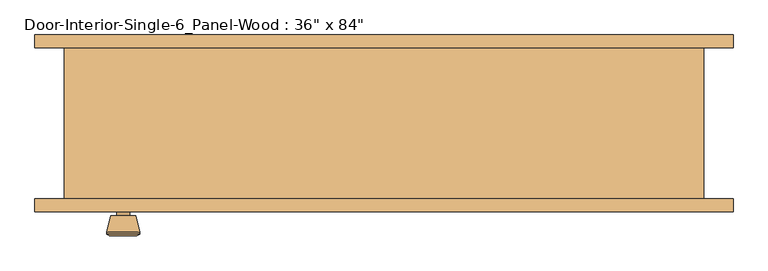
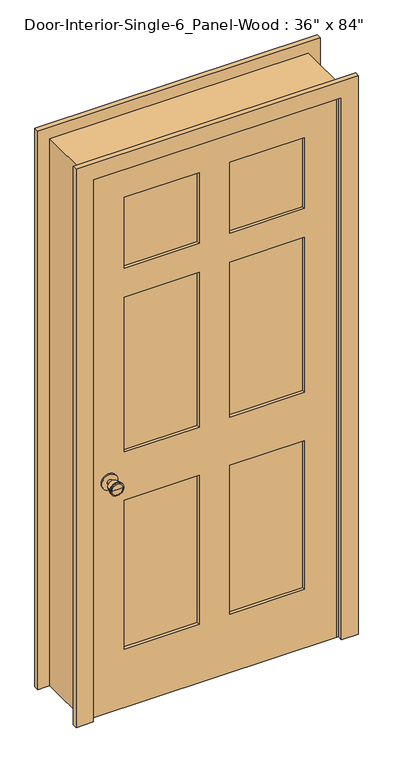
"""IFC4 building model written with IfcOpenShell, lengths in millimetres: door geometry."""

from ifc_helpers import new_model, si_unit, point, frame, frame_2d, origin, place, context, project, spatial, polyline, circle_curve, trimmed, segment, composite_curve, outline, extrude, faceted_brep, source, transform, mapped, element, save
from ifc_brep_helpers import plane_surface, cylinder_surface, revolved_surface, advanced_brep


def door_c5239341(model_context):
    return source(origin(), model_context, "Body", "SolidModel", [
        advanced_brep(
        [(-393.7, -70.2, 914.4), (-403.7, -70.2, 914.4), (-383.7, -70.2, 914.4), (-373.2241324, -21.2, 914.4), (-414.1758676, -21.2, 914.4), (-393.7, -21.2, 914.4), (-368.7, -23.0278681, 914.4), (-418.7, -23.0278681, 914.4), (-368.7, -26.4915463, 914.4), (-418.7, -26.4915463, 914.4), (-375.063764, -51.2, 914.4), (-412.336236, -51.2, 914.4), (-383.7, -51.2, 914.4), (-403.7, -51.2, 914.4)],
        [
            (0, 1),
            (1, 2, circle_curve(frame((-393.7, -70.2, 914.4), z_axis=(0.0, -1.0, 0.0), x_axis=(-1.0, 0.0, 0.0)), 10.0)),
            (2, 0),
            (2, 1, circle_curve(frame((-393.7, -70.2, 914.4), z_axis=(0.0, -1.0, 0.0), x_axis=(-1.0, 0.0, 0.0)), 10.0)),
            (3, 4, circle_curve(frame((-393.7, -21.2, 914.4), z_axis=(0.0, 1.0, 0.0), x_axis=(-1.0, 0.0, 0.0)), 20.4758676)),
            (4, 5),
            (5, 3),
            (4, 3, circle_curve(frame((-393.7, -21.2, 914.4), z_axis=(0.0, 1.0, 0.0), x_axis=(-1.0, 0.0, 0.0)), 20.4758676)),
            (6, 7, circle_curve(frame((-393.7, -23.0278681, 914.4), z_axis=(0.0, 1.0, 0.0), x_axis=(-1.0, 0.0, 0.0)), 25.0)),
            (7, 4),
            (3, 6),
            (7, 6, circle_curve(frame((-393.7, -23.0278681, 914.4), z_axis=(0.0, 1.0, 0.0), x_axis=(-1.0, 0.0, 0.0)), 25.0)),
            (8, 9, circle_curve(frame((-393.7, -26.4915463, 914.4), z_axis=(0.0, 1.0, 0.0), x_axis=(-1.0, 0.0, 0.0)), 25.0)),
            (9, 7),
            (6, 8),
            (9, 8, circle_curve(frame((-393.7, -26.4915463, 914.4), z_axis=(0.0, 1.0, 0.0), x_axis=(-1.0, 0.0, 0.0)), 25.0)),
            (10, 11, circle_curve(frame((-393.7, -51.2, 914.4), z_axis=(0.0, 1.0, 0.0), x_axis=(-1.0, 0.0, 0.0)), 18.636236)),
            (11, 9),
            (8, 10),
            (11, 10, circle_curve(frame((-393.7, -51.2, 914.4), z_axis=(0.0, 1.0, 0.0), x_axis=(-1.0, 0.0, 0.0)), 18.636236)),
            (12, 13, circle_curve(frame((-393.7, -51.2, 914.4), z_axis=(0.0, 1.0, 0.0), x_axis=(-1.0, 0.0, 0.0)), 10.0)),
            (13, 11),
            (10, 12),
            (13, 12, circle_curve(frame((-393.7, -51.2, 914.4), z_axis=(0.0, 1.0, 0.0), x_axis=(-1.0, 0.0, 0.0)), 10.0)),
            (1, 13),
            (12, 2),
        ],
        [
            plane_surface(frame((-393.7, -70.2, 914.4), z_axis=(0.0, -1.0, 0.0), x_axis=(-1.0, 0.0, 0.0))),
            plane_surface(frame((-393.7, -21.2, 914.4), z_axis=(0.0, 1.0, 0.0), x_axis=(-1.0, 0.0, 0.0))),
            revolved_surface(polyline([(-414.1758676, -21.2, 914.4), (-418.7, -23.0278681, 914.4)]), (-393.7, -70.2, 914.4), (0.0, -1.0, 0.0)),
            cylinder_surface(frame((-393.7, -70.2, 914.4), z_axis=(0.0, -1.0, 0.0), x_axis=(-1.0, 0.0, 0.0)), 25.0),
            revolved_surface(polyline([(-418.7, -26.4915463, 914.4), (-412.336236, -51.2, 914.4)]), (-393.7, -70.2, 914.4), (0.0, -1.0, 0.0)),
            plane_surface(frame((-393.7, -51.2, 914.4), z_axis=(0.0, -1.0, 0.0), x_axis=(-1.0, 0.0, 0.0))),
            cylinder_surface(frame((-393.7, -70.2, 914.4), z_axis=(0.0, -1.0, 0.0), x_axis=(-1.0, 0.0, 0.0)), 10.0),
        ],
        [
            (0, [[1, 2, 3]]),
            (0, [[-3, 4, -1]]),
            (1, [[5, 6, 7]]),
            (1, [[8, -7, -6]]),
            (2, [[9, 10, -5, 11]]),
            (2, [[12, -11, -8, -10]]),
            (3, [[13, 14, -9, 15]]),
            (3, [[16, -15, -12, -14]]),
            (4, [[17, 18, -13, 19]]),
            (4, [[20, -19, -16, -18]]),
            (5, [[21, 22, -17, 23]]),
            (5, [[24, -23, -20, -22]]),
            (6, [[-2, 25, -21, 26]]),
            (6, [[-4, -26, -24, -25]]),
        ],
    ),
        extrude(outline(composite_curve([segment(trimmed(circle_curve(frame_2d((914.4, -393.7)), 30.0), [point((914.4, -423.7))], [point((914.4, -363.7))], False, "CARTESIAN"), True, "CONTINUOUS"), segment(trimmed(circle_curve(frame_2d((914.4, -393.7)), 30.0), [point((914.4, -363.7))], [point((914.4, -423.7))], False, "CARTESIAN"), True, "CONTINUOUS")], self_intersect=False)), frame((0.0, -76.2, 0.0), z_axis=(0.0, 1.0, 0.0), x_axis=(0.0, 0.0, 1.0)), (0.0, 0.0, 1.0), 6.0),
        advanced_brep(
        [(-393.7, -117.125, 914.4), (-383.7, -117.125, 914.4), (-403.7, -117.125, 914.4), (-373.2241324, -166.125, 914.4), (-393.7, -166.125, 914.4), (-414.1758676, -166.125, 914.4), (-368.7, -164.2971319, 914.4), (-418.7, -164.2971319, 914.4), (-368.7, -160.8334537, 914.4), (-418.7, -160.8334537, 914.4), (-375.063764, -136.125, 914.4), (-412.336236, -136.125, 914.4), (-383.7, -136.125, 914.4), (-403.7, -136.125, 914.4)],
        [
            (0, 1),
            (1, 2, circle_curve(frame((-393.7, -117.125, 914.4), z_axis=(0.0, 1.0, 0.0), x_axis=(-1.0, 0.0, 0.0)), 10.0)),
            (2, 0),
            (2, 1, circle_curve(frame((-393.7, -117.125, 914.4), z_axis=(0.0, 1.0, 0.0), x_axis=(-1.0, 0.0, 0.0)), 10.0)),
            (3, 4),
            (4, 5),
            (5, 3, circle_curve(frame((-393.7, -166.125, 914.4), z_axis=(0.0, -1.0, 0.0), x_axis=(-1.0, 0.0, 0.0)), 20.4758676)),
            (3, 5, circle_curve(frame((-393.7, -166.125, 914.4), z_axis=(0.0, -1.0, 0.0), x_axis=(-1.0, 0.0, 0.0)), 20.4758676)),
            (6, 3),
            (5, 7),
            (7, 6, circle_curve(frame((-393.7, -164.2971319, 914.4), z_axis=(0.0, -1.0, 0.0), x_axis=(-1.0, 0.0, 0.0)), 25.0)),
            (6, 7, circle_curve(frame((-393.7, -164.2971319, 914.4), z_axis=(0.0, -1.0, 0.0), x_axis=(-1.0, 0.0, 0.0)), 25.0)),
            (8, 6),
            (7, 9),
            (9, 8, circle_curve(frame((-393.7, -160.8334537, 914.4), z_axis=(0.0, -1.0, 0.0), x_axis=(-1.0, 0.0, 0.0)), 25.0)),
            (8, 9, circle_curve(frame((-393.7, -160.8334537, 914.4), z_axis=(0.0, -1.0, 0.0), x_axis=(-1.0, 0.0, 0.0)), 25.0)),
            (10, 8),
            (9, 11),
            (11, 10, circle_curve(frame((-393.7, -136.125, 914.4), z_axis=(0.0, -1.0, 0.0), x_axis=(-1.0, 0.0, 0.0)), 18.636236)),
            (10, 11, circle_curve(frame((-393.7, -136.125, 914.4), z_axis=(0.0, -1.0, 0.0), x_axis=(-1.0, 0.0, 0.0)), 18.636236)),
            (12, 10),
            (11, 13),
            (13, 12, circle_curve(frame((-393.7, -136.125, 914.4), z_axis=(0.0, -1.0, 0.0), x_axis=(-1.0, 0.0, 0.0)), 10.0)),
            (12, 13, circle_curve(frame((-393.7, -136.125, 914.4), z_axis=(0.0, -1.0, 0.0), x_axis=(-1.0, 0.0, 0.0)), 10.0)),
            (1, 12),
            (13, 2),
        ],
        [
            plane_surface(frame((-393.7, -117.125, 914.4), z_axis=(0.0, 1.0, 0.0), x_axis=(-1.0, 0.0, 0.0))),
            plane_surface(frame((-393.7, -166.125, 914.4), z_axis=(0.0, -1.0, 0.0), x_axis=(-1.0, 0.0, 0.0))),
            revolved_surface(polyline([(-414.1758676, -166.125, 914.4), (-418.7, -164.2971319, 914.4)]), (-393.7, -117.125, 914.4), (0.0, 1.0, 0.0)),
            cylinder_surface(frame((-393.7, -117.125, 914.4), z_axis=(0.0, 1.0, 0.0), x_axis=(-1.0, 0.0, 0.0)), 25.0),
            revolved_surface(polyline([(-418.7, -160.8334537, 914.4), (-412.336236, -136.125, 914.4)]), (-393.7, -117.125, 914.4), (0.0, 1.0, 0.0)),
            plane_surface(frame((-393.7, -136.125, 914.4), z_axis=(0.0, 1.0, 0.0), x_axis=(-1.0, 0.0, 0.0))),
            cylinder_surface(frame((-393.7, -117.125, 914.4), z_axis=(0.0, 1.0, 0.0), x_axis=(-1.0, 0.0, 0.0)), 10.0),
        ],
        [
            (0, [[1, 2, 3]]),
            (0, [[-3, 4, -1]]),
            (1, [[5, 6, 7]]),
            (1, [[-6, -5, 8]]),
            (2, [[9, -7, 10, 11]]),
            (2, [[-10, -8, -9, 12]]),
            (3, [[13, -11, 14, 15]]),
            (3, [[-14, -12, -13, 16]]),
            (4, [[17, -15, 18, 19]]),
            (4, [[-18, -16, -17, 20]]),
            (5, [[21, -19, 22, 23]]),
            (5, [[-22, -20, -21, 24]]),
            (6, [[25, -23, 26, -2]]),
            (6, [[-26, -24, -25, -4]]),
        ],
    ),
        extrude(outline(composite_curve([segment(trimmed(circle_curve(frame_2d((914.4, -393.7)), 30.0), [point((914.4, -423.7))], [point((914.4, -363.7))], False, "CARTESIAN"), True, "CONTINUOUS"), segment(trimmed(circle_curve(frame_2d((914.4, -393.7)), 30.0), [point((914.4, -363.7))], [point((914.4, -423.7))], False, "CARTESIAN"), True, "CONTINUOUS")], self_intersect=False)), frame((0.0, -117.125, 0.0), z_axis=(0.0, 1.0, 0.0), x_axis=(0.0, 0.0, 1.0)), (0.0, 0.0, 1.0), 6.0),
        faceted_brep([(482.6, -111.125, 0.0), (457.2, -111.125, 0.0), (457.2, -76.2, 0.0), (444.5, -76.2, 0.0), (444.5, -41.275, 0.0), (457.2, -41.275, 0.0), (457.2, 117.475, 0.0), (482.6, 117.475, 0.0), (482.6, 117.475, 2159.0), (482.6, -111.125, 2159.0), (457.2, 117.475, 2133.6), (-457.2, 117.475, 2133.6), (-457.2, 117.475, 0.0), (-482.6, 117.475, 0.0), (-482.6, 117.475, 2159.0), (457.2, -41.275, 2133.6), (444.5, -41.275, 2120.9), (-444.5, -41.275, 2120.9), (-444.5, -41.275, 0.0), (-457.2, -41.275, 0.0), (-457.2, -41.275, 2133.6), (444.5, -76.2, 2120.9), (457.2, -76.2, 2133.6), (-457.2, -76.2, 2133.6), (-457.2, -76.2, 0.0), (-444.5, -76.2, 0.0), (-444.5, -76.2, 2120.9), (457.2, -111.125, 2133.6), (-482.6, -111.125, 2159.0), (-482.6, -111.125, 0.0), (-457.2, -111.125, 0.0), (-457.2, -111.125, 2133.6)], [[[0, 1, 2, 3, 4, 5, 6, 7]], [[7, 8, 9, 0]], [[6, 10, 11, 12, 13, 14, 8, 7]], [[5, 15, 10, 6]], [[4, 16, 17, 18, 19, 20, 15, 5]], [[3, 21, 16, 4]], [[2, 22, 23, 24, 25, 26, 21, 3]], [[1, 27, 22, 2]], [[0, 9, 28, 29, 30, 31, 27, 1]], [[8, 14, 28, 9]], [[15, 20, 11, 10]], [[21, 26, 17, 16]], [[27, 31, 23, 22]], [[29, 13, 12, 19, 18, 25, 24, 30]], [[14, 13, 29, 28]], [[20, 19, 12, 11]], [[26, 25, 18, 17]], [[31, 30, 24, 23]]]),
        extrude(outline(polyline([(2133.6, -457.2), (0.0, -457.2), (0.0, 457.2), (2133.6, 457.2), (2133.6, -457.2)]), holes=[polyline([(2014.5375, 57.15), (2014.5375, 336.55), (1735.1375, 336.55), (1735.1375, 57.15), (2014.5375, 57.15)]), polyline([(1620.8375, 336.55), (1009.65, 336.55), (1009.65, 57.15), (1620.8375, 57.15), (1620.8375, 336.55)]), polyline([(1009.65, -57.15), (1009.65, -336.55), (1620.8375, -336.55), (1620.8375, -57.15), (1009.65, -57.15)]), polyline([(1735.1375, -336.55), (2014.5375, -336.55), (2014.5375, -57.15), (1735.1375, -57.15), (1735.1375, -336.55)]), polyline([(819.15, 57.15), (819.15, 336.55), (231.775, 336.55), (231.775, 57.15), (819.15, 57.15)]), polyline([(231.775, -57.15), (231.775, -336.55), (819.15, -336.55), (819.15, -57.15), (231.775, -57.15)])]), frame((0.0, -111.125, 0.0), z_axis=(0.0, 1.0, 0.0), x_axis=(0.0, 0.0, 1.0)), (0.0, 0.0, 1.0), 34.925),
        extrude(outline(polyline([(336.55, -87.8416667), (336.55, -99.4833333), (57.15, -99.4833333), (57.15, -87.8416667), (336.55, -87.8416667)])), frame((0.0, 0.0, 1735.1375), z_axis=(0.0, 0.0, 1.0), x_axis=(1.0, 0.0, 0.0)), (0.0, 0.0, 1.0), 279.4),
        extrude(outline(polyline([(336.55, -87.8416667), (336.55, -99.4833333), (57.15, -99.4833333), (57.15, -87.8416667), (336.55, -87.8416667)])), frame((0.0, 0.0, 1009.65), z_axis=(0.0, 0.0, 1.0), x_axis=(1.0, 0.0, 0.0)), (0.0, 0.0, 1.0), 611.1875),
        extrude(outline(polyline([(-57.15, -87.8416667), (-57.15, -99.4833333), (-336.55, -99.4833333), (-336.55, -87.8416667), (-57.15, -87.8416667)])), frame((0.0, 0.0, 1009.65), z_axis=(0.0, 0.0, 1.0), x_axis=(1.0, 0.0, 0.0)), (0.0, 0.0, 1.0), 611.1875),
        extrude(outline(polyline([(-57.15, -87.8416667), (-57.15, -99.4833333), (-336.55, -99.4833333), (-336.55, -87.8416667), (-57.15, -87.8416667)])), frame((0.0, 0.0, 1735.1375), z_axis=(0.0, 0.0, 1.0), x_axis=(1.0, 0.0, 0.0)), (0.0, 0.0, 1.0), 279.4),
        extrude(outline(polyline([(336.55, -87.8416667), (336.55, -99.4833333), (57.15, -99.4833333), (57.15, -87.8416667), (336.55, -87.8416667)])), frame((0.0, 0.0, 231.775), z_axis=(0.0, 0.0, 1.0), x_axis=(1.0, 0.0, 0.0)), (0.0, 0.0, 1.0), 587.375),
        extrude(outline(polyline([(-57.15, -87.8416667), (-57.15, -99.4833333), (-336.55, -99.4833333), (-336.55, -87.8416667), (-57.15, -87.8416667)])), frame((0.0, 0.0, 231.775), z_axis=(0.0, 0.0, 1.0), x_axis=(1.0, 0.0, 0.0)), (0.0, 0.0, 1.0), 587.375),
        extrude(outline(polyline([(0.0, 527.05), (2203.45, 527.05), (2203.45, -527.05), (0.0, -527.05), (0.0, -463.55), (2139.95, -463.55), (2139.95, 463.55), (0.0, 463.55), (0.0, 527.05)])), frame((0.0, -130.175, 0.0), z_axis=(0.0, 1.0, 0.0), x_axis=(0.0, 0.0, 1.0)), (0.0, 0.0, 1.0), 19.05),
        extrude(outline(polyline([(0.0, 527.05), (2203.45, 527.05), (2203.45, -527.05), (0.0, -527.05), (0.0, -463.55), (2139.95, -463.55), (2139.95, 463.55), (0.0, 463.55), (0.0, 527.05)])), frame((0.0, 117.475, 0.0), z_axis=(0.0, 1.0, 0.0), x_axis=(0.0, 0.0, 1.0)), (0.0, 0.0, 1.0), 19.05),
    ])


if __name__ == "__main__":
    model = new_model("IFC4")
    model_context = context("Model", 3, world=origin())
    ifc_project = project(units=[si_unit("LENGTHUNIT", "METRE", prefix="MILLI")], contexts=[model_context])
    site = spatial("IfcSite", under=ifc_project)
    building = spatial("IfcBuilding", under=site)
    placement = place(None, origin())
    door_shape = door_c5239341(model_context)
    element("IfcDoor", 1, ObjectType="Door-Interior-Single-6_Panel-Wood : 36\" x 84\"", at=placement, inside=building, context=model_context, shape_type="MappedRepresentation", body=[
        mapped(door_shape, transform((0.0, 0.0, 0.0), x_axis=(1.0, 0.0, 0.0), y_axis=(0.0, 1.0, 0.0), z_axis=(0.0, 0.0, 1.0))),
    ])
    save(model, "model.ifc")

# Revit data of these elements
# Type "Door-Interior-Single-6_Panel-Wood : 36\" x 84\""
#   Type Mark = "8"
#   Assembly Code = "C1020300"
#   Analytic Construction = "Wooden"
#   Top Rail = 0' - 4 11/16"
#   Top Panel = 0' - 11"
#   Thickness = 0' - 1 3/8"
#   Thermal Resistance (R) = 2.5876 (h·ft²·°F)/BTU
#   Swing Angle [instance default] = 90.00°
#   Stiles = 0' - 4 3/4"
#   Rough Width = 3' - 2"
#   Rough Height = 7' - 1"
#   Mullion = 0' - 4 1/2"
#   Lock Rail = 0' - 7 1/2"
#   Intermediate Rail = 0' - 4 1/2"
#   Height = 7' - 0"
#   Width = 3' - 0"
#   Heat Transfer Coefficient (U) = 0.3865 BTU/(h·ft²·°F)
#   Bottom Rail = 0' - 9 1/8"
#   Trim Material = Cherry
#   Panel Material = Cherry
#   Frame Material = Cherry
#   Door Handle Material = Aluminum
#   Visual Light Transmittance = 0
#   Solar Heat Gain Coefficient = 0
#   Wall Closure = (empty or 0)
#   Function = (empty or 0)
# Element 1 (IfcDoor, "Door-Interior-Single-6_Panel-Wood : 36\" x 84\"")
#   Materials on its faces: "Cherry", "Aluminum"
# Materials
#   "Cherry": class "Wood", colour RGB 226 177 128, transparency 0, Description = "Prunus Serotina", Cost = 0
#   "Aluminum": class "Metal", colour RGB 247 247 247, transparency 0, Description = "Aluminum 6061", Cost = 0
